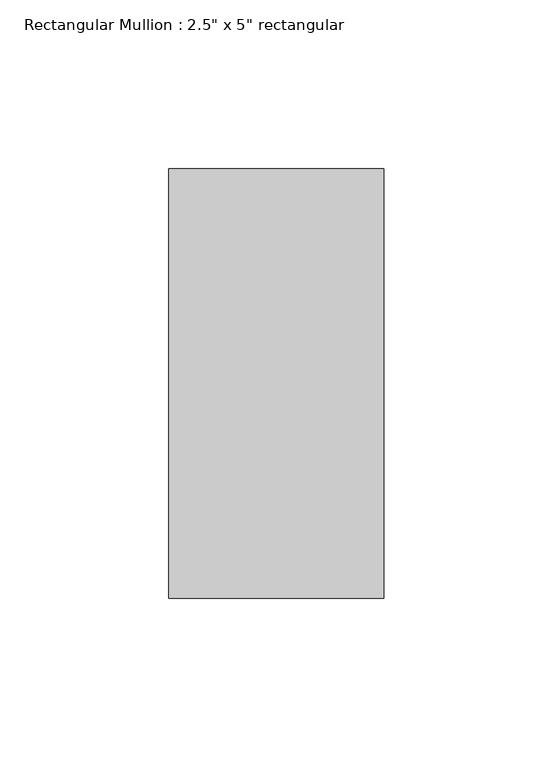
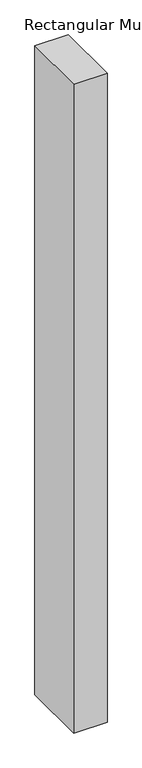
"""IFC4 building model written with IfcOpenShell, lengths in millimetres: member geometry."""

from ifc_helpers import new_model, si_unit, frame, origin, place, context, project, spatial, polyline, outline, extrude, source, transform, mapped, element, save


def member_19a13f65(model_context):
    return source(origin(), model_context, "Body", "SweptSolid", [
        extrude(outline(polyline([(0.0, 63.5), (0.0, -63.5), (-63.5, -63.5), (-63.5, 63.5), (0.0, 63.5)])), frame((0.0, 0.0, -1301.6187331), z_axis=(0.0, 0.0, 1.0), x_axis=(1.0, 0.0, 0.0)), (0.0, 0.0, 1.0), 1301.6187331),
    ])


if __name__ == "__main__":
    model = new_model("IFC4")
    model_context = context("Model", 3, world=origin())
    ifc_project = project(units=[si_unit("LENGTHUNIT", "METRE", prefix="MILLI")], contexts=[model_context])
    site = spatial("IfcSite", under=ifc_project)
    building = spatial("IfcBuilding", under=site)
    placement = place(None, origin())
    member_shape = member_19a13f65(model_context)
    element("IfcMember", 1, ObjectType="Rectangular Mullion : 2.5\" x 5\" rectangular", at=placement, inside=building, context=model_context, shape_type="MappedRepresentation", body=[
        mapped(member_shape, transform((0.0, 0.0, 0.0), x_axis=(1.0, 0.0, 0.0), y_axis=(0.0, 1.0, 0.0), z_axis=(0.0, 0.0, 1.0))),
    ])
    save(model, "model.ifc")

# Revit data of these elements
# Type "Rectangular Mullion : 2.5\" x 5\" rectangular"
#   built-in parameter 1007304 = 0.416667 (stored number, unit not read)
#   built-in parameter 1007301 = 0.104167 (stored number, unit not read)
#   built-in parameter 1007300 = 0.104167 (stored number, unit not read)
# Element 1 (IfcMember, "Rectangular Mullion : 2.5\" x 5\" rectangular")
#   Materials on its faces: "Aluminum"
# Materials
#   "Aluminum": class "Metal", colour RGB 247 247 247, transparency 0, Description = "Aluminum 6061", Cost = 0
